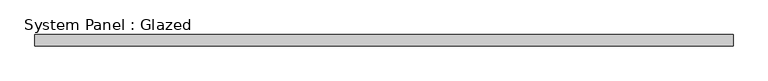
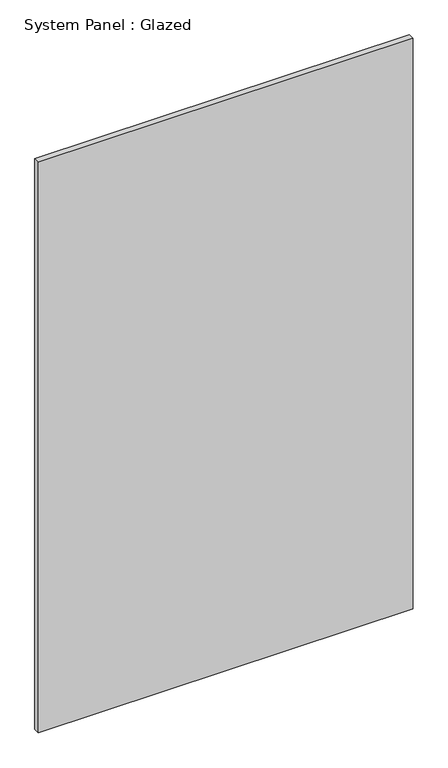
"""IFC4 building model written with IfcOpenShell, lengths in millimetres: plate geometry, System Panel : Glazed."""

from ifc_helpers import new_model, si_unit, origin, origin_with_axes, place, context, project, spatial, polyline, outline, extrude, source, transform, mapped, element, save


def system_panel_glazed_8270a400(model_context):
    return source(origin(), model_context, "Body", "SweptSolid", [
        extrude(outline(polyline([(787.4, 19.05), (-787.4, 19.05), (-787.4, 44.45), (787.4, 44.45), (787.4, 19.05)])), origin_with_axes(), (0.0, 0.0, 1.0), 2535.3380434),
    ])


if __name__ == "__main__":
    model = new_model("IFC4")
    model_context = context("Model", 3, world=origin())
    ifc_project = project(units=[si_unit("LENGTHUNIT", "METRE", prefix="MILLI")], contexts=[model_context])
    site = spatial("IfcSite", under=ifc_project)
    building = spatial("IfcBuilding", under=site)
    placement = place(None, origin())
    system_panel_glazed_shape = system_panel_glazed_8270a400(model_context)
    element("IfcPlate", 1, ObjectType="System Panel : Glazed", at=placement, inside=building, context=model_context, shape_type="MappedRepresentation", body=[
        mapped(system_panel_glazed_shape, transform((0.0, 0.0, 0.0), x_axis=(1.0, 0.0, 0.0), y_axis=(0.0, 1.0, 0.0), z_axis=(0.0, 0.0, 1.0))),
    ])
    save(model, "model.ifc")

# Revit data of these elements
# Type "System Panel : Glazed"
#   Construction Type Id = "GSP4R"
#   Analytic Construction = "1/8 in Pilkington single glazing"
#   Visual Light Transmittance = 0.9
#   Solar Heat Gain Coefficient = 0.86
#   Heat Transfer Coefficient (U) = 1.18115 BTU/(h·ft²·°F)
# Element 1 (IfcPlate, "System Panel : Glazed")
#   Materials on its faces: "Glass"
# Materials
#   "Glass": class "Glass", colour RGB 0 128 192, transparency 0.75, Description = "Soda Lime Glass", Cost = 0
